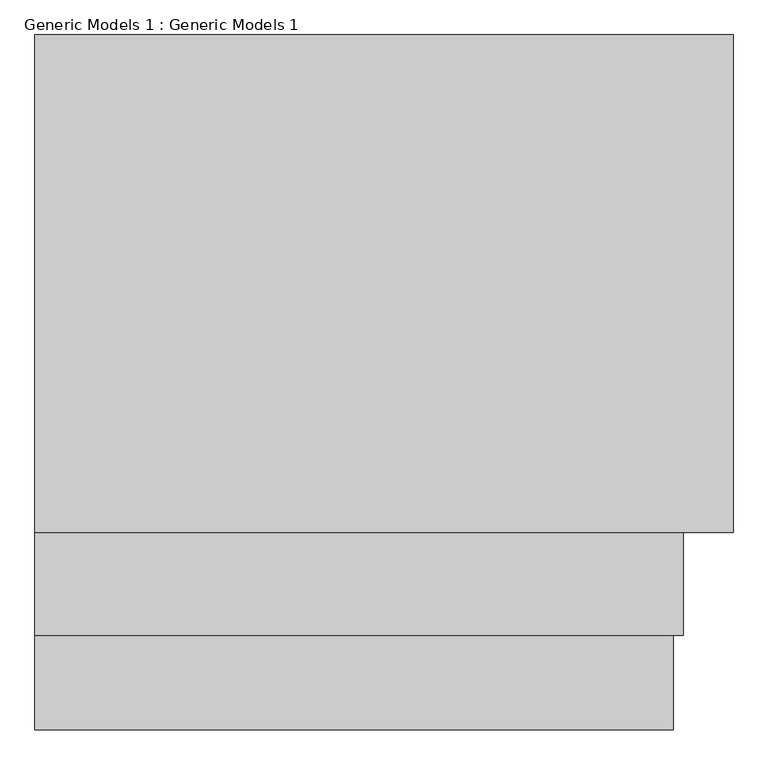
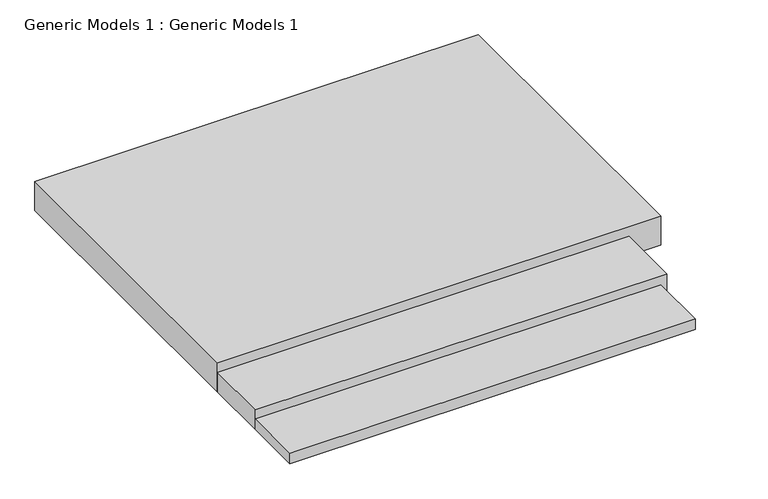
"""IFC4 building model written with IfcOpenShell, lengths in millimetres: proxy geometry, Generic Models 1 : Generic Models 1."""

from ifc_helpers import new_model, si_unit, origin, origin_with_axes, place, context, project, spatial, polyline, outline, extrude, source, transform, mapped, element, save


def generic_models_1_generic_models_1_906a804f(model_context):
    return source(origin(), model_context, "Body", "SweptSolid", [
        extrude(outline(polyline([(-17235.5161422, -15094.7171312), (-21617.0161422, -15094.7171312), (-21617.0161422, -11970.5171312), (-17235.5161422, -11970.5171312), (-17235.5161422, -15094.7171312)])), origin_with_axes(), (0.0, 0.0, 1.0), 304.8),
        extrude(outline(polyline([(-17610.2339948, -16333.949459), (-21617.0161422, -16333.949459), (-21617.0161422, -15742.2978151), (-17610.2339948, -15742.2978151), (-17610.2339948, -16333.949459)])), origin_with_axes(), (0.0, 0.0, 1.0), 108.6151429),
        extrude(outline(polyline([(-17549.7093594, -15742.2978151), (-21617.0161422, -15742.2978151), (-21617.0161422, -15094.7171312), (-17549.7093594, -15094.7171312), (-17549.7093594, -15742.2978151)])), origin_with_axes(), (0.0, 0.0, 1.0), 203.2),
    ])


if __name__ == "__main__":
    model = new_model("IFC4")
    model_context = context("Model", 3, world=origin())
    ifc_project = project(units=[si_unit("LENGTHUNIT", "METRE", prefix="MILLI")], contexts=[model_context])
    site = spatial("IfcSite", under=ifc_project)
    building = spatial("IfcBuilding", under=site)
    placement = place(None, origin())
    generic_models_1_generic_models_1_shape = generic_models_1_generic_models_1_906a804f(model_context)
    element("IfcBuildingElementProxy", 1, Name="Generic Models 1 : Generic Models 1", ObjectType="Generic Models 1 : Generic Models 1", at=placement, inside=building, context=model_context, shape_type="MappedRepresentation", body=[
        mapped(generic_models_1_generic_models_1_shape, transform((0.0, 0.0, 0.0), x_axis=(1.0, 0.0, 0.0), y_axis=(0.0, 1.0, 0.0), z_axis=(0.0, 0.0, 1.0))),
    ])
    save(model, "model.ifc")
